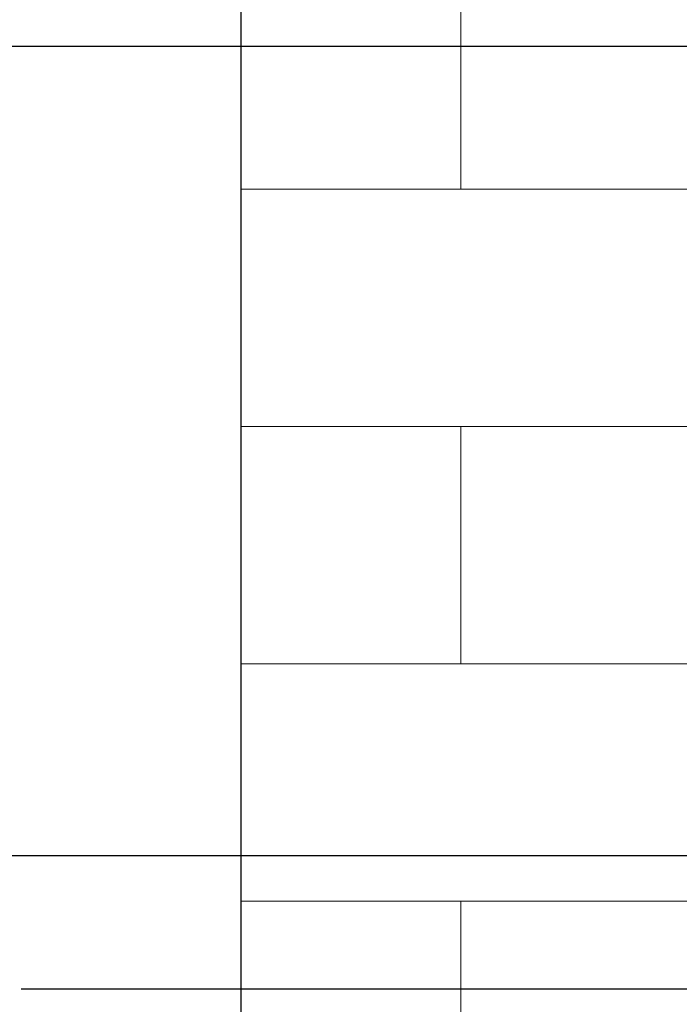
# Model space of a CAD drawing. Units: inches. Extents: x 37 to 824, y -700 to 234.
# Tile 15 of 77: x 348 to 378, y -581 to -536. Entities that reach past the tile are written whole.
import ezdxf

# ---------------------------------------------------------------- set-up
doc = ezdxf.new("R2010")
doc.units = ezdxf.units.IN
doc.header["$MEASUREMENT"] = 0
for name, color, linetype, lineweight in [('A-ANNO-DIMS', 2, 'Continuous', 18), ('A-ELEV', 3, 'Continuous', 25), ('A-ELEV-PATT', 8, 'Continuous', 13)]:
    doc.layers.add(name, color=color, linetype=linetype, lineweight=lineweight)
doc.styles.get("Standard").update_dxf_attribs({"font": 'arial.ttf'})
doc.dimstyles.get("Standard").update_dxf_attribs({"dimtxt": 0.18, "dimasz": 0.18, "dimexe": 0.18, "dimexo": 0.0625, "dimgap": 0.09, "dimtad": 0, "dimtih": 1, "dimtoh": 1, "dimdec": 1, "dimzin": 0, "dimdsep": 46, "dimlunit": 4, "dimtxsty": 'Standard', "dimcen": 0.09, "dimadec": 0, "dimazin": 0, "dimtfac": 1, "dimtdec": 1, "dimtofl": 0, "dimtmove": 0, "dimatfit": 3, "dimfxl": 1, "dimtolj": 1, "dimtzin": 0, "dimarcsym": 0})

# ---------------------------------------------------------------- blocks, each defined once
blk = doc.blocks.new('*D28')
at = {"layer": 'A-ANNO-DIMS', "color": 0, "lineweight": -2, "ltscale": 0.5, "transparency": 16777216}
for p, q in [((255.14, -537.627), (449.868, -537.627)), ((449.688, -543.627), (449.688, -558.537)), ((449.688, -579.627), (449.688, -564.717)), ((294.64, -585.627), (449.868, -585.627))]:
    blk.add_line(p, q, dxfattribs=at)
at = {"layer": 'A-ANNO-DIMS', "color": 0, "ltscale": 0.5, "transparency": 16777216}
for points in [[(448.688, -543.627), (450.688, -543.627), (449.688, -537.627)], [(448.688, -579.627), (450.688, -579.627), (449.688, -585.627)]]:
    blk.add_solid(points, dxfattribs=at)
at = {"layer": 'Defpoints', "color": 0, "ltscale": 0.5, "transparency": 16777216}
for p in [(255.077, -537.627), (294.577, -585.627), (449.688, -585.627)]:
    blk.add_point(p, dxfattribs=at)
at = {"layer": 'A-ANNO-DIMS', "color": 0, "ltscale": 0.5, "transparency": 16777216, "insert": (449.688, -561.627), "char_height": 6, "attachment_point": 5}
blk.add_mtext("\\A1;4'", dxfattribs=at)
blk = doc.blocks.new('*D31')
at = {"layer": 'A-ANNO-DIMS', "color": 0, "lineweight": -2, "ltscale": 0.5, "transparency": 16777216}
for p, q in [((255.14, -489.627), (449.772, -489.627)), ((449.592, -495.627), (449.592, -510.537)), ((449.592, -531.627), (449.592, -516.717)), ((255.14, -537.627), (449.772, -537.627))]:
    blk.add_line(p, q, dxfattribs=at)
at = {"layer": 'A-ANNO-DIMS', "color": 0, "ltscale": 0.5, "transparency": 16777216}
for points in [[(448.592, -495.627), (450.592, -495.627), (449.592, -489.627)], [(448.592, -531.627), (450.592, -531.627), (449.592, -537.627)]]:
    blk.add_solid(points, dxfattribs=at)
at = {"layer": 'Defpoints', "color": 0, "ltscale": 0.5, "transparency": 16777216}
for p in [(255.077, -489.627), (449.592, -489.627), (255.077, -537.627)]:
    blk.add_point(p, dxfattribs=at)
at = {"layer": 'A-ANNO-DIMS', "color": 0, "ltscale": 0.5, "transparency": 16777216, "insert": (449.592, -513.627), "char_height": 6, "attachment_point": 5}
blk.add_mtext("\\A1;4'", dxfattribs=at)
blk = doc.blocks.new('*D101')
at = {"layer": 'A-ANNO-DIMS', "color": 0, "lineweight": -2, "ltscale": 0.5, "transparency": 16777216}
for p, q in [((348.258, -496.007), (556.923, -496.007)), ((556.743, -496.187), (556.743, -537.825)), ((556.743, -579.827), (556.743, -538.189)), ((348.258, -580.007), (556.923, -580.007))]:
    blk.add_line(p, q, dxfattribs=at)
at = {"layer": 'A-ANNO-DIMS', "color": 0, "ltscale": 0.5, "transparency": 16777216}
for points in [[(556.713, -496.187), (556.773, -496.187), (556.743, -496.007)], [(556.713, -579.827), (556.773, -579.827), (556.743, -580.007)]]:
    blk.add_solid(points, dxfattribs=at)
at = {"layer": 'Defpoints', "color": 0, "ltscale": 0.5, "transparency": 16777216}
for p in [(348.196, -496.007), (348.196, -580.007), (556.743, -580.007)]:
    blk.add_point(p, dxfattribs=at)
at = {"layer": 'A-ANNO-DIMS', "color": 0, "ltscale": 0.5, "transparency": 16777216, "insert": (556.743, -538.007), "char_height": 0.18, "attachment_point": 5}
blk.add_mtext('\\A1;7\'-0"', dxfattribs=at)
blk = doc.blocks.new('*D104')
at = {"layer": 'A-ANNO-DIMS', "color": 0, "lineweight": -2, "ltscale": 0.5, "transparency": 16777216}
for p, q in [((341.258, -505.03), (556.923, -505.03)), ((556.743, -505.21), (556.743, -539.336)), ((556.743, -573.827), (556.743, -539.7)), ((341.258, -574.007), (556.923, -574.007))]:
    blk.add_line(p, q, dxfattribs=at)
at = {"layer": 'A-ANNO-DIMS', "color": 0, "ltscale": 0.5, "transparency": 16777216}
for points in [[(556.713, -505.21), (556.773, -505.21), (556.743, -505.03)], [(556.713, -573.827), (556.773, -573.827), (556.743, -574.007)]]:
    blk.add_solid(points, dxfattribs=at)
at = {"layer": 'Defpoints', "color": 0, "ltscale": 0.5, "transparency": 16777216}
for p in [(341.196, -505.03), (341.196, -574.007), (556.743, -574.007)]:
    blk.add_point(p, dxfattribs=at)
at = {"layer": 'A-ANNO-DIMS', "color": 0, "ltscale": 0.5, "transparency": 16777216, "insert": (556.743, -539.518), "char_height": 0.18, "attachment_point": 5}
blk.add_mtext('\\A1;5\'-9"', dxfattribs=at)

msp = doc.modelspace()

# ---------------------------------------------------------------- hatches: boundary and pattern name
at = {"layer": 'A-ELEV-PATT', "ltscale": 0.5}
h = msp.add_hatch(dxfattribs=at)
h.set_pattern_fill('AR-BRSTD', color=256, scale=4)
h.paths.add_polyline_path([(299.077, -489.627), (358.132, -489.627), (358.132, -585.627), (428.077, -585.627), (428.077, -465.627), (161.077, -465.627), (161.077, -585.627), (299.077, -585.627)])
h.paths.add_polyline_path([(205.077, -537.627), (205.077, -489.627), (255.077, -489.627), (255.077, -537.627)], flags=16)

# ---------------------------------------------------------------- linework, layer by layer
at = {"layer": 'A-ELEV', "ltscale": 0.5}
msp.add_lwpolyline([(299.077, -489.627), (358.132, -489.627), (358.132, -585.627), (299.077, -585.627)], close=True, dxfattribs=at)

# ---------------------------------------------------------------- dimensions: what is measured, and where the dimension line sits
at = {"layer": 'A-ANNO-DIMS', "ltscale": 0.5}
for base, p1, p2, override, picture, middle in [((449.592, -489.627), (255.077, -537.627), (255.077, -489.627), {"dimtxt": 6, "dimasz": 6, "dimclrd": 0, "dimclre": 0, "dimclrt": 0}, '*D31', (449.592, -513.627)), ((556.743, -580.007), (348.196, -496.007), (348.196, -580.007), {"dimdec": 1, "dimlfac": 1, "dimrnd": 0, "dimzin": 1, "dimdsep": 46, "dimlunit": 4, "dimfrac": 2}, '*D101', (556.743, -538.007)), ((556.743, -574.007), (341.196, -505.03), (341.196, -574.007), {"dimdec": 1, "dimlfac": 1, "dimrnd": 0, "dimzin": 1, "dimdsep": 46, "dimlunit": 4, "dimfrac": 2}, '*D104', (556.743, -539.518)), ((449.688, -585.627), (255.077, -537.627), (294.577, -585.627), {"dimtxt": 6, "dimasz": 6, "dimclrd": 0, "dimclre": 0, "dimclrt": 0}, '*D28', (449.688, -561.627))]:
    dim = msp.add_linear_dim(base=base, p1=p1, p2=p2, angle=90, dimstyle='Standard', override=override, dxfattribs=at)
    dim.commit()
    dim.dimension.update_dxf_attribs({"geometry": picture, "text_midpoint": middle})

doc.saveas('drawing.dxf')
